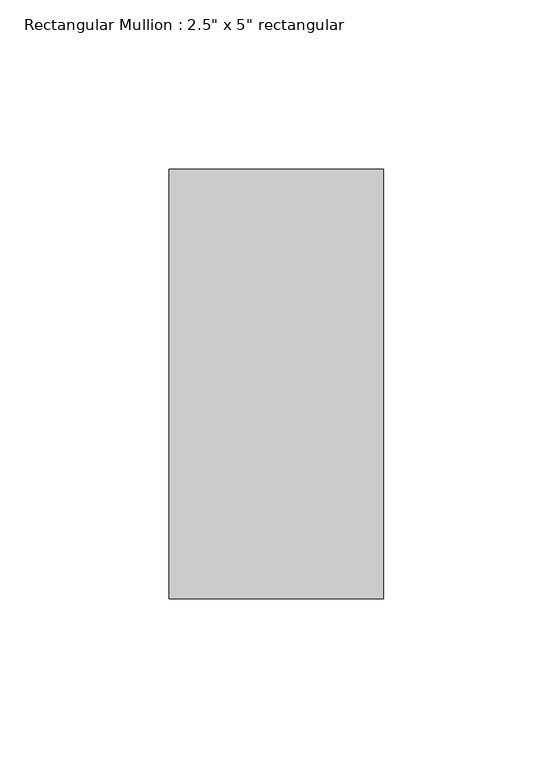
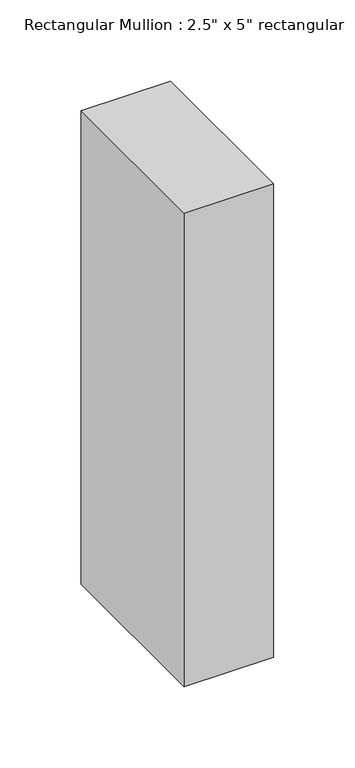
"""IFC4 building model written with IfcOpenShell, lengths in millimetres: member geometry."""

from ifc_helpers import new_model, si_unit, frame, origin, place, context, project, spatial, polyline, outline, extrude, source, transform, mapped, element, save


def member_ffcd2ccf(model_context):
    return source(origin(), model_context, "Body", "SweptSolid", [
        extrude(outline(polyline([(0.0, 63.5), (0.0, -63.5), (-63.5, -63.5), (-63.5, 63.5), (0.0, 63.5)])), frame((0.0, 0.0, -355.6), z_axis=(0.0, 0.0, 1.0), x_axis=(1.0, 0.0, 0.0)), (0.0, 0.0, 1.0), 355.6),
    ])


if __name__ == "__main__":
    model = new_model("IFC4")
    model_context = context("Model", 3, world=origin())
    ifc_project = project(units=[si_unit("LENGTHUNIT", "METRE", prefix="MILLI")], contexts=[model_context])
    site = spatial("IfcSite", under=ifc_project)
    building = spatial("IfcBuilding", under=site)
    placement = place(None, origin())
    member_shape = member_ffcd2ccf(model_context)
    element("IfcMember", 1, ObjectType="Rectangular Mullion : 2.5\" x 5\" rectangular", at=placement, inside=building, context=model_context, shape_type="MappedRepresentation", body=[
        mapped(member_shape, transform((0.0, 0.0, 0.0), x_axis=(1.0, 0.0, 0.0), y_axis=(0.0, 1.0, 0.0), z_axis=(0.0, 0.0, 1.0))),
    ])
    save(model, "model.ifc")

# Revit data of these elements
# Type "Rectangular Mullion : 2.5\" x 5\" rectangular"
#   built-in parameter 1007304 = 0.416667 (stored number, unit not read)
#   built-in parameter 1007301 = 0.104167 (stored number, unit not read)
#   built-in parameter 1007300 = 0.104167 (stored number, unit not read)
# Element 1 (IfcMember, "Rectangular Mullion : 2.5\" x 5\" rectangular")
#   Materials on its faces: "door colour"
# Materials
#   "door colour": class "Generic", colour RGB 120 120 120, transparency 0, Cost = 0
